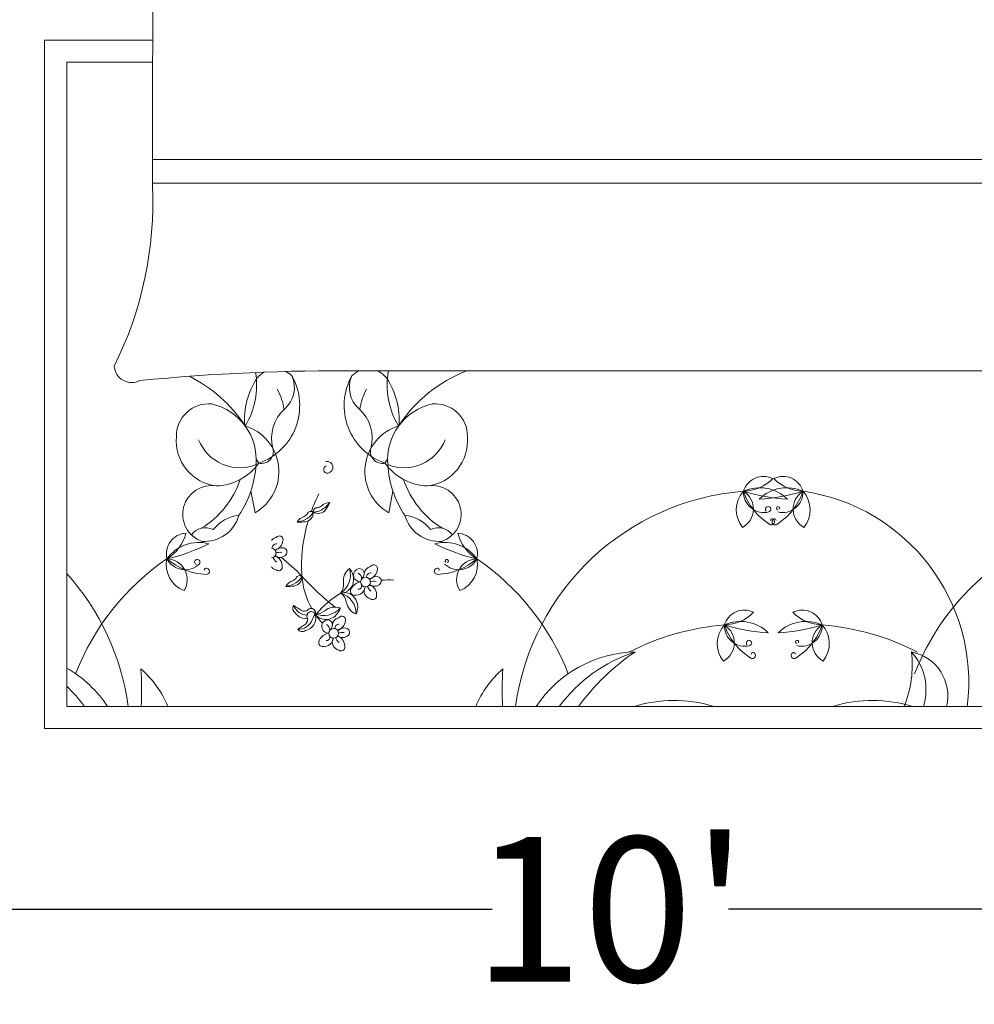
# Model space of a CAD drawing. Units: inches. Extents: x 0 to 281, y -535 to 46.
# Tile 15 of 22: x 72 to 112, y -77 to -36. Entities that reach past the tile are written whole.
import ezdxf

# ---------------------------------------------------------------- set-up
doc = ezdxf.new("R2010")
doc.units = ezdxf.units.IN
doc.header["$MEASUREMENT"] = 0
doc.layers.add('A-ANNO-DIMS', color=2, linetype='Continuous', lineweight=18)
doc.layers.add('A-FURN', color=8, linetype='Continuous', lineweight=18)
doc.styles.get("Standard").update_dxf_attribs({"font": 'arial.ttf'})
doc.dimstyles.get("Standard").update_dxf_attribs({"dimtxt": 0.18, "dimasz": 0.18, "dimexe": 0.18, "dimexo": 0.0625, "dimgap": 0.09, "dimtad": 0, "dimtih": 1, "dimtoh": 1, "dimdec": 0, "dimzin": 0, "dimdsep": 46, "dimlunit": 3, "dimtxsty": 'Standard', "dimcen": 0.09, "dimadec": 0, "dimazin": 0, "dimtfac": 1, "dimtdec": 0, "dimtofl": 0, "dimtmove": 0, "dimatfit": 3, "dimfxl": 1, "dimtolj": 1, "dimtzin": 0, "dimarcsym": 0})

# ---------------------------------------------------------------- blocks, each defined once
blk = doc.blocks.new('*D2')
at = {"layer": 'A-ANNO-DIMS', "color": 0, "lineweight": -2, "transparency": 16777216}
for p, q in [((36.459, -73.027), (36.459, -72.91)), ((156.459, -73.027), (156.459, -72.91)), ((36.639, -73.09), (91.56, -73.09)), ((156.279, -73.09), (101.358, -73.09))]:
    blk.add_line(p, q, dxfattribs=at)
at = {"layer": 'A-ANNO-DIMS', "color": 0, "transparency": 16777216}
for points in [[(36.639, -73.06), (36.639, -73.12), (36.459, -73.09)], [(156.279, -73.06), (156.279, -73.12), (156.459, -73.09)]]:
    blk.add_solid(points, dxfattribs=at)
at = {"layer": 'Defpoints', "color": 0, "transparency": 16777216}
for p in [(36.459, -73.09), (156.459, -73.09), (156.459, -73.09)]:
    blk.add_point(p, dxfattribs=at)
at = {"layer": 'A-ANNO-DIMS', "color": 0, "transparency": 16777216, "insert": (96.459, -73.09), "char_height": 6, "attachment_point": 5}
blk.add_mtext("\\A1;10'", dxfattribs=at)

msp = doc.modelspace()

# ---------------------------------------------------------------- linework, layer by layer
at = {"layer": 'A-FURN'}
for p, q in [((73.019, -37.076), (77.499, -37.076)), ((73.019, -65.604), (73.019, -37.076)), ((77.497, -37.994), (73.937, -37.994)), ((73.937, -37.994), (73.937, -64.686)), ((126.28, -42.015), (77.493, -42.015)), ((126.355, -43.003), (77.492, -43.003)), ((118.239, -50.782), (86.086, -50.782)), ((81.741, -56.657), (81.566, -55.762)), ((87.275, -56.657), (87.451, -55.762)), ((73.937, -64.686), (129.836, -64.686)), ((130.754, -65.604), (73.019, -65.604))]:
    msp.add_line(p, q, dxfattribs=at)
msp.add_lwpolyline([(77.53, -28.07, 0.001242), (77.492, -43.096, -0.127202), (75.905, -50.584)], format="xyb", dxfattribs=at)
for centre in [(86.316, -59.527), (84.997, -61.653)]:
    msp.add_circle(centre, 0.202, dxfattribs=at)
for centre, radius, start, end in [((76.634, -50.533), 0.731, 183.98, 297.3412), ((85.141, -133.217), 82.44, 89.34325, 95.68869), ((78.523, -51.368), 3.281, 328.8218, 9.1554), ((82.587, -51.658), 0.954, 120.0293, 142.325), ((81.064, -52.22), 2.524, 289.2822, 29.1751), ((82.184, -51.469), 1.185, 311.5653, 23.8354), ((82.587, -51.658), 0.954, 44.4517, 63.558), ((87.952, -52.22), 2.524, 150.8249, 250.7178), ((86.832, -51.469), 1.185, 156.1646, 228.4347), ((86.429, -51.658), 0.954, 113.229, 135.5483), ((86.429, -51.658), 0.954, 37.675, 66.7144), ((90.493, -51.368), 3.281, 169.7133, 211.1782), ((92.691, -56.359), 5.994, 111.4941, 146.3329), ((76.325, -56.359), 5.994, 33.6671, 63.2997), ((84.358, -52.792), 3.054, 145.785, 184.7304), ((84.658, -52.792), 3.054, 355.2696, 34.215), ((80.683, -52.677), 2.276, 7.436, 29.9149), ((88.333, -52.677), 2.276, 150.0851, 172.564), ((79.817, -53.481), 1.337, 84.4856, 181.0538), ((79.406, -54.47), 2.382, 355.2933, 76.921), ((89.61, -54.47), 2.382, 103.079, 184.7067), ((89.2, -53.481), 1.337, 358.9462, 95.5144), ((84.047, -53.57), 1.624, 131.5653, 195.1471), ((84.969, -53.57), 1.624, 344.8529, 48.4347), ((80.759, -54.95), 1.969, 299.9085, 73.1337), ((88.257, -54.95), 1.969, 106.8663, 240.0915), ((80.365, -53.672), 1.892, 174.9449, 262.8857), ((81.109, -52.955), 1.838, 201.5819, 291.4221), ((87.908, -52.955), 1.838, 248.5779, 338.4181), ((88.651, -53.672), 1.892, 277.1143, 5.0551), ((82.006, -54.123), 0.492, 257.3041, 15.1471), ((87.01, -54.123), 0.492, 164.8529, 282.6959), ((80.036, -53.252), 2.3, 272.3591, 324.0401), ((77.538, -54.407), 4.25, 326.2883, 356.5076), ((84.358, -52.792), 3.054, 212.7011, 216.3445), ((84.718, -54.775), 0.248, 280.4384, 100.4136), ((84.658, -52.792), 3.054, 323.6555, 327.2989), ((88.98, -53.252), 2.3, 215.9599, 267.6409), ((91.478, -54.407), 4.25, 183.4924, 213.7117), ((84.735, -54.869), 0.153, 102.7051, 280.4384), ((77.573, -54.105), 3.739, 301.2614, 341.7045), ((91.443, -54.105), 3.739, 198.2955, 238.7386), ((102.797, -56.009), 0.857, 63.0274, 163.8037), ((101.929, -54.004), 1.766, 271.4585, 315.3727), ((103.615, -56.009), 0.857, 16.1963, 116.9726), ((104.484, -54.004), 1.766, 224.6273, 268.5415), ((79.929, -56.721), 1.188, 80.264, 250.8688), ((90.225, -58.855), 6.559, 153.0032, 159.8941), ((89.087, -56.721), 1.188, 289.1312, 99.736), ((102.778, -66.079), 10.341, 94.4623, 172.255), ((102.823, -56.54), 1.147, 137.7873, 219.1145), ((101.521, -56.505), 0.864, 298.5391, 58.3627), ((102.819, -55.803), 0.846, 177.7585, 283.852), ((102.647, -57.259), 1.635, 45.5411, 114.3101), ((104.138, -48.866), 7.235, 252.593, 267.2582), ((104.448, -54.922), 2.615, 198.9159, 238.011), ((103.766, -57.259), 1.635, 65.6899, 134.4589), ((102.275, -48.866), 7.235, 272.7418, 287.407), ((101.965, -54.922), 2.615, 301.989, 341.0841), ((103.593, -55.803), 0.846, 256.148, 2.2415), ((104.892, -56.505), 0.864, 121.6373, 241.4609), ((103.589, -56.54), 1.147, 320.8855, 42.2127), ((103.3, -63.692), 8.004, 352.8636, 81.8197), ((84.818, -56.655), 0.416, 87.3579, 140.4944), ((83.857, -55.461), 1.252, 301.164, 321.5612), ((82.839, -55.242), 2.233, 324.6898, 333.4936), ((82.992, -55.82), 1.272, 308.2101, 316.3071), ((83.773, -56.656), 0.38, 278.3432, 4.2869), ((83.563, -56.323), 0.664, 300.656, 332.6341), ((84.061, -56.761), 0.161, 55.7657, 157.4417), ((84.312, -56.611), 0.161, 84.3784, 186.0543), ((84.161, -55.964), 0.664, 269.1859, 301.164), ((84.356, -56.307), 0.38, 237.5332, 323.4768), ((83.988, -55.224), 1.272, 285.5129, 293.6099), ((102.995, -56.515), 0.112, 283.852, 219.9245), ((103.407, -56.472), 0.0674, 320.1909, 256.0209), ((79.644, -56.364), 1.484, 265.969, 344.3045), ((81.243, -58.337), 1.581, 96.1662, 141.5825), ((83.861, -57.228), 0.416, 101.3256, 154.4621), ((83.263, -55.817), 1.252, 280.2588, 300.656), ((83.551, -54.816), 2.233, 268.3264, 277.1302), ((90.225, -58.855), 6.559, 163.5842, 183.8277), ((87.773, -58.337), 1.581, 38.4175, 83.8338), ((89.372, -56.364), 1.484, 195.6955, 274.031), ((103.13, -57.031), 0.128, 238.011, 71.5592), ((103.151, -56.968), 0.0624, 71.5592, 188.0167), ((103.282, -57.031), 0.128, 108.4408, 301.989), ((103.261, -56.968), 0.0624, 351.9833, 108.4408), ((78.923, -58.364), 0.857, 92.9516, 193.728), ((77.17, -57.06), 1.766, 301.3827, 345.2969), ((79.685, -58.009), 0.728, 63.9755, 143.2681), ((89.331, -58.009), 0.728, 36.7319, 116.0245), ((90.094, -58.364), 0.857, 346.272, 87.0484), ((91.846, -57.06), 1.766, 194.7031, 238.6173), ((79.416, -59.523), 1.635, 75.4653, 144.2343), ((82.685, -58.016), 0.336, 101.5637, 142.6358), ((82.415, -57.752), 0.485, 288.7263, 352.5032), ((82.745, -57.776), 0.156, 345.2356, 144.9248), ((89.6, -59.523), 1.635, 35.7657, 104.5347), ((76.522, -51.505), 7.235, 282.5173, 297.1824), ((82.406, -58.328), 0.202, 273.2768, 86.7232), ((82.641, -58.137), 0.193, 91.1081, 181.8675), ((82.846, -58.525), 0.417, 80.3487, 133.6538), ((82.767, -58.958), 0.66, 83.0852, 105.7171), ((82.887, -58.285), 0.174, 317.6792, 80.3487), ((92.494, -51.505), 7.235, 242.8176, 257.4827), ((83.93, -67.102), 10.341, 124.3865, 158.5908), ((79.21, -58.812), 1.147, 167.7115, 249.0387), ((78.064, -59.431), 0.864, 328.4633, 88.2869), ((79.811, -56.599), 2.615, 228.8402, 267.9352), ((78.839, -58.175), 0.846, 207.6827, 313.7762), ((79.347, -58.705), 0.112, 313.7762, 249.7183), ((83.04, -58.258), 0.612, 203.4276, 227.6104), ((82.771, -58.18), 0.33, 229.7889, 317.6792), ((82.399, -58.879), 0.469, 355.053, 68.3618), ((78.195, -64.435), 7.519, 43.1541, 52.0459), ((89.205, -56.599), 2.615, 272.0648, 311.1598), ((90.177, -58.175), 0.846, 226.2238, 332.3173), ((89.682, -58.662), 0.0674, 290.2667, 226.2271), ((90.952, -59.431), 0.864, 91.7131, 211.5367), ((89.806, -58.812), 1.147, 290.9613, 12.2885), ((85.086, -67.102), 10.341, 21.4092, 55.6135), ((118.687, -67.102), 10.341, 124.3865, 158.5908), ((79.708, -59.019), 0.0624, 101.4834, 217.9409), ((79.722, -59.084), 0.128, 267.9352, 101.4834), ((82.681, -58.702), 0.333, 217.7621, 259.0403), ((82.712, -58.906), 0.155, 232.4737, 355.053), ((84.772, -59.227), 0.919, 304.5369, 16.3699), ((86.048, -59.485), 0.65, 127.3105, 187.9252), ((85.155, -59.412), 0.668, 355.0106, 41.658), ((86.093, -59.246), 0.275, 126.1046, 271.4281), ((86.063, -59.171), 0.198, 353.7526, 131.7054), ((86.595, -59.214), 0.336, 101.5637, 176.365), ((86.551, -59.336), 0.193, 91.1081, 181.8675), ((86.325, -58.951), 0.485, 288.7263, 352.5032), ((86.655, -58.974), 0.156, 345.2356, 144.9248), ((89.295, -59.084), 0.128, 78.5166, 272.0648), ((89.308, -59.019), 0.0624, 322.0591, 78.5166), ((66.238, -66.079), 10.341, 7.745, 41.8856), ((83.389, -59.892), 0.416, 101.3256, 154.4621), ((82.791, -58.482), 1.252, 280.2588, 300.656), ((82.52, -58.485), 1.272, 308.2101, 316.3071), ((83.301, -59.321), 0.38, 278.3432, 4.2869), ((83.091, -58.987), 0.664, 300.656, 332.6341), ((83.589, -59.426), 0.161, 55.7657, 157.4417), ((86.957, -59.02), 3.288, 184.756, 209.2041), ((91.691, -52.018), 10.821, 222.2412, 232.1744), ((85.263, -59.432), 0.559, 272.8499, 356.1226), ((86.262, -60.136), 0.636, 104.7558, 148.0499), ((85.877, -59.406), 0.278, 0.0645, 61.1507), ((85.943, -59.17), 0.317, 311.8413, 355.7877), ((86.756, -59.723), 0.417, 80.3487, 133.6538), ((86.676, -60.157), 0.66, 83.0852, 105.7171), ((86.796, -59.484), 0.174, 317.6792, 80.3487), ((87.295, -63.387), 3.944, 87.1071, 94.7585), ((83.079, -57.481), 2.233, 268.3264, 277.1302), ((84.868, -59.649), 0.541, 321.7607, 7.9252), ((85.422, -60.522), 0.559, 20.5253, 88.5375), ((85.892, -59.905), 0.2, 148.0499, 225.6268), ((87.295, -63.387), 3.944, 113.0501, 113.8477), ((85.905, -59.681), 0.398, 247.4086, 351.4386), ((86.017, -59.697), 0.134, 262.906, 7.132), ((86.591, -59.9), 0.333, 151.2196, 259.0403), ((86.95, -59.457), 0.612, 203.4276, 227.6104), ((86.681, -59.378), 0.33, 229.7889, 317.6792), ((86.309, -60.077), 0.469, 355.053, 68.3618), ((87.295, -63.387), 3.944, 120.544, 139.818), ((84.982, -60.427), 0.541, 8.7227, 54.8872), ((85.011, -60.859), 0.919, 0.278, 72.111), ((86.16, -60.246), 0.65, 188.7227, 249.3375), ((85.325, -60.572), 0.668, 334.9899, 21.6373), ((86.622, -60.104), 0.155, 232.4737, 355.053), ((83.529, -60.622), 0.225, 146.8636, 236.9021), ((86.704, -55.661), 5.892, 235.1882, 238.8844), ((83.916, -60.295), 0.61, 199.4799, 267.6828), ((83.78, -60.506), 0.233, 238.8844, 314.2646), ((84.065, -60.931), 0.176, 19.3605, 201.7548), ((84.066, -60.799), 0.176, 311.8703, 134.2646), ((84.577, -60.002), 0.919, 247.2305, 319.0635), ((84.273, -60.311), 0.541, 264.4544, 310.6188), ((85.049, -61.216), 0.65, 70.0041, 130.6188), ((84.628, -60.424), 0.668, 297.7043, 344.3516), ((102.005, -61.548), 0.857, 63.0274, 163.8037), ((101.137, -59.543), 1.766, 271.4585, 315.3727), ((104.407, -61.548), 0.857, 16.1963, 116.9726), ((105.276, -59.543), 1.766, 224.6273, 268.5415), ((83.848, -60.526), 0.525, 212.8155, 277.3992), ((83.542, -60.877), 0.61, 266.9701, 338.2913), ((83.729, -61.028), 0.525, 280.3057, 17.1958), ((83.685, -61.082), 0.233, 306.3746, 21.7548), ((87.372, -62.402), 3.513, 153.7819, 158.2913), ((86.957, -59.02), 3.288, 214.0033, 222.4917), ((84.669, -60.526), 0.559, 218.3208, 298.8162), ((84.774, -61.372), 0.275, 126.1046, 271.4281), ((84.744, -61.297), 0.198, 353.7526, 131.7054), ((85.276, -61.34), 0.336, 101.5637, 176.365), ((85.006, -61.077), 0.485, 288.7263, 352.5032), ((85.336, -61.1), 0.156, 345.2356, 144.9248), ((101.855, -62.798), 1.635, 45.5411, 114.3101), ((104.557, -62.798), 1.635, 65.6899, 134.4589), ((80.329, -56.526), 5.892, 302.6784, 306.3746), ((83.696, -61.359), 0.225, 214.3538, 304.3923), ((84.558, -61.532), 0.278, 0.0645, 61.1507), ((84.624, -61.296), 0.317, 311.8413, 355.7877), ((85.232, -61.462), 0.193, 91.1081, 181.8675), ((85.436, -61.849), 0.417, 80.3487, 133.6538), ((85.477, -61.609), 0.174, 317.6792, 80.3487), ((101.987, -71.619), 10.341, 94.4623, 117.4146), ((102.031, -62.079), 1.147, 137.7873, 219.1145), ((100.729, -62.044), 0.864, 298.5391, 58.3627), ((102.027, -61.342), 0.846, 177.7585, 283.852), ((103.656, -60.461), 2.615, 198.9159, 238.011), ((103.346, -54.405), 7.235, 252.593, 267.2582), ((103.066, -54.405), 7.235, 272.7418, 287.407), ((102.756, -60.461), 2.615, 301.989, 341.0841), ((104.385, -61.342), 0.846, 256.148, 2.2415), ((105.684, -62.044), 0.864, 121.6373, 241.4609), ((104.381, -62.079), 1.147, 320.8855, 42.2127), ((104.426, -71.619), 10.341, 62.5854, 85.5377), ((84.573, -62.031), 0.2, 148.0499, 225.6268), ((84.943, -62.262), 0.636, 104.7558, 148.0499), ((84.586, -61.806), 0.398, 247.4086, 351.4386), ((84.698, -61.823), 0.134, 262.906, 7.132), ((85.272, -62.026), 0.333, 151.2196, 259.0403), ((85.631, -61.582), 0.612, 203.4276, 227.6104), ((85.362, -61.504), 0.33, 229.7889, 317.6792), ((84.99, -62.203), 0.469, 355.053, 68.3618), ((85.357, -62.282), 0.66, 83.0852, 105.7171), ((102.203, -62.054), 0.112, 283.852, 219.9245), ((104.199, -62.011), 0.0674, 320.1909, 256.0209), ((85.302, -62.23), 0.155, 232.4737, 355.053), ((97.59, -67.464), 5.039, 91.272, 146.5383), ((99.403, -68.404), 6.28, 107.8504, 143.6964), ((102.704, -70.169), 9.341, 124.0123, 144.053), ((102.339, -62.57), 0.128, 238.011, 71.5592), ((102.36, -62.507), 0.0624, 71.5592, 188.0167), ((104.074, -62.57), 0.128, 108.4408, 301.989), ((104.053, -62.507), 0.0624, 351.9833, 108.4408), ((104.335, -62.96), 4.63, 338.117, 6.6195), ((108.582, -64.249), 1.856, 346.3898, 79.0739), ((107.187, -63.994), 2.347, 342.8609, 41.9049), ((71.426, -67.464), 5.039, 33.4617, 60.1116), ((74.248, -66.299), 4.205, 22.5547, 48.9546), ((62.73, -64.039), 14.308, 357.4081, 3.6519), ((94.768, -66.299), 4.205, 131.0454, 157.4453), ((106.286, -64.039), 14.308, 176.3481, 182.5919), ((69.613, -68.404), 6.28, 36.3036, 46.4814), ((99.094, -70.123), 5.686, 73.5431, 107.0202), ((107.318, -70.123), 5.686, 72.9798, 106.4569), ((101.347, -73.054), 8.409, 94.3787, 95.6357), ((105.776, -78.815), 15.027, 109.7217, 109.9028), ((105.065, -73.054), 8.409, 84.3643, 85.6213), ((100.636, -78.815), 15.027, 70.0972, 70.2783)]:
    msp.add_arc(centre, radius, start, end, dxfattribs=at)

# ---------------------------------------------------------------- dimensions: what is measured, and where the dimension line sits
at = {"layer": 'A-ANNO-DIMS'}
dim = msp.add_linear_dim(base=(156.459, -73.09), p1=(36.459, -73.09), p2=(156.459, -73.09), dimstyle='Standard', override={"dimtxt": 6, "dimclrd": 0, "dimclre": 0, "dimclrt": 0}, dxfattribs=at)
dim.commit()
dim.dimension.update_dxf_attribs({"geometry": '*D2', "text_midpoint": (96.459, -73.09)})

doc.saveas('drawing.dxf')
